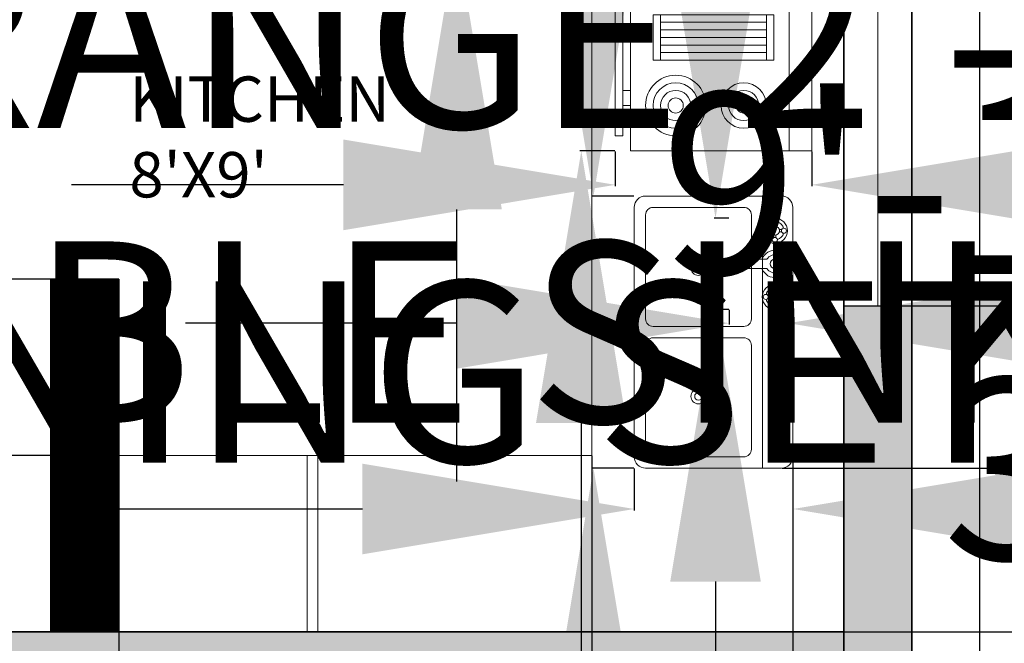
# Model space of a CAD drawing. Units: inches. Extents: x 2838 to 4029, y 1041 to 1915.
# Tile 9 of 16: x 3510 to 3640, y 1377 to 1460. Entities that reach past the tile are written whole.
import ezdxf

# ---------------------------------------------------------------- set-up
doc = ezdxf.new("R2010")
doc.units = ezdxf.units.IN
doc.header["$MEASUREMENT"] = 0
for name, color, linetype, lineweight in [('A-ANNO-DIMS', 2, 'Continuous', 18), ('A-AREA-IDEN', 7, 'Continuous', 18), ('A-EQPM', 8, 'Continuous', 18), ('A-FLOR', 7, 'Continuous', 25), ('A-FLOR-CASE', 8, 'Continuous', 18), ('A-FLOR-FIXT', 9, 'Continuous', 18), ('A-GLAZ', 4, 'Continuous', 18), ('A-WALL', 7, 'Continuous', 35), ('A-WALL-PATT', 252, 'Continuous', 13)]:
    doc.layers.add(name, color=color, linetype=linetype, lineweight=lineweight)
doc.styles.get("Standard").update_dxf_attribs({"font": 'arial.ttf'})
doc.dimstyles.get("Standard").update_dxf_attribs({"dimtxt": 24, "dimasz": 36, "dimexe": 0.18, "dimexo": 0.0625, "dimgap": 0.09, "dimtad": 0, "dimtih": 1, "dimtoh": 1, "dimdec": 0, "dimzin": 0, "dimdsep": 46, "dimlunit": 3, "dimtxsty": 'Standard', "dimcen": 0.09, "dimadec": 0, "dimazin": 0, "dimtfac": 1, "dimtdec": 0, "dimtofl": 0, "dimtmove": 0, "dimatfit": 3, "dimfxl": 1, "dimtolj": 1, "dimtzin": 0, "dimarcsym": 0})

# ---------------------------------------------------------------- blocks, each defined once
blk = doc.blocks.new('Faucet - Bathroom top')
for p, q in [((-4.107, 0.125), (-4.375, 0.125)), ((-3.75, 0.4788), (-3.75, 0.75)), ((-3.5, 0.482), (-3.5, 0.75)), ((-3.1461, 0.125), (-2.875, 0.125)), ((3.143, 0.125), (2.875, 0.125)), ((3.5, 0.4788), (3.5, 0.75)), ((3.75, 0.482), (3.75, 0.75)), ((4.1039, 0.125), (4.375, 0.125)), ((-4.1039, -0.125), (-4.375, -0.125)), ((-3.75, -0.4821), (-3.75, -0.75)), ((-3.5, -0.4789), (-3.5, -0.75)), ((-3.143, -0.125), (-2.875, -0.125)), ((-0.5, -0.8639), (-0.5, -4.5)), ((0.5, -4.5), (0.5, -0.8631)), ((3.1461, -0.125), (2.875, -0.125)), ((3.5, -0.4821), (3.5, -0.75)), ((3.75, -0.4789), (3.75, -0.75)), ((4.107, -0.125), (4.375, -0.125))]:
    blk.add_line(p, q)
for centre, radius in [((-3.625, 0), 1.375), ((-3.625, 1), 0.2795), ((3.625, 0), 1.375), ((3.625, 1), 0.2795), ((-4.625, 0), 0.2795), ((-3.625, 0), 0.5), ((-2.625, 0), 0.2795), ((0, 0), 0.5), ((2.625, 0), 0.2795), ((3.625, 0), 0.5), ((4.625, 0), 0.2795), ((-3.625, -1), 0.2795), ((3.625, -1), 0.2795)]:
    blk.add_circle(centre, radius)
for centre, radius, start, end in [((0, 0), 1.5, 289.6514, 250.3603), ((-3.625, 0), 1, 105.2407, 164.2093), ((-3.625, 0), 1, 16.44125, 74.07887), ((0, 0), 1, 300.3431, 239.7554), ((3.625, 0), 1, 106.12, 164.0884), ((3.625, 0), 1, 16.23422, 73.90469), ((-3.625, 0), 1, 196.2342, 253.9047), ((-3.625, 0), 1, 286.12, 344.0884), ((3.625, 0), 1, 196.4413, 254.0789), ((3.625, 0), 1, 285.2407, 344.2093), ((0, -4.5), 0.5, 180, 0)]:
    blk.add_arc(centre, radius, start, end)
blk = doc.blocks.new('Range-Oven - 30 in top')
for p, q in [((0, -3), (30, -3)), ((12, -6), (18, -6)), ((13, -20), (13, -6)), ((14, -6), (14, -20)), ((15, -20), (15, -6)), ((16, -6), (16, -20)), ((17, -20), (17, -6)), ((18, -20), (12, -20)), ((6, -24), (6, -25)), ((8, -25), (8, -24)), ((22, -25), (22, -24)), ((24, -24), (24, -25))]:
    blk.add_line(p, q)
for points in [[(0, -24), (0, 0), (30, 0), (30, -24)], [(12, -21), (12, -5), (18, -5), (18, -21)], [(2, -26), (2, -25), (28, -25), (28, -26)]]:
    blk.add_lwpolyline(points, close=True)
for centre, radius in [((6, -9), 4), ((6, -9), 3), ((24, -9), 3), ((6, -9), 2), ((24, -9), 2), ((6, -9), 1), ((24, -9), 1), ((24, -18), 4), ((6, -18), 3), ((24, -18), 3), ((6, -18), 2), ((24, -18), 2), ((6, -18), 1), ((24, -18), 1)]:
    blk.add_circle(centre, radius)
blk = doc.blocks.new('Sink-double - 36 in top')
for p, q in [((-18, -4), (18, -4)), ((-0.75, -18.5), (-0.75, -6.5)), ((0.75, -6.5), (0.75, -18.5))]:
    blk.add_line(p, q)
for points in [[(-16.5, 0), (16.5, 0)], [(-18, -19.5), (-18, -1.5)], [(18, -1.5), (18, -19.5)], [(-16.5, -18.5), (-16.5, -6.5)], [(-15.5, -5.5), (-1.75, -5.5)], [(1.75, -5.5), (15.5, -5.5)], [(16.5, -6.5), (16.5, -18.5)], [(-1.75, -19.5), (-15.5, -19.5)], [(15.5, -19.5), (1.75, -19.5)], [(16.5, -21), (-16.5, -21)]]:
    blk.add_lwpolyline(points)
for centre, radius in [((-8.5, -12.5), 1), ((8.5, -12.5), 1), ((-8.5, -12.5), 0.5), ((8.5, -12.5), 0.5)]:
    blk.add_circle(centre, radius)
for centre, radius, start, end in [((-16.5, -1.5), 1.5, 90, 180), ((16.5, -1.5), 1.5, 0, 90), ((-15.5, -6.5), 1, 90, 180), ((-1.75, -6.5), 1, 0, 90), ((1.75, -6.5), 1, 90, 180), ((15.5, -6.5), 1, 0, 90), ((-16.5, -19.5), 1.5, 180, 270), ((-15.5, -18.5), 1, 180, 270), ((-1.75, -18.5), 1, 270, 0), ((1.75, -18.5), 1, 180, 270), ((15.5, -18.5), 1, 270, 0), ((16.5, -19.5), 1.5, 270, 0)]:
    blk.add_arc(centre, radius, start, end)
blk = doc.blocks.new('*D17')
at = {"layer": 'A-ANNO-DIMS', "color": 0, "lineweight": -2, "transparency": 16777216}
for p, q in [((3627.79, 1671.3), (3713.18, 1671.3)), ((3713, 1635.3), (3713, 1443.64)), ((3713, 1227.3), (3713, 1418.95)), ((3627.79, 1191.3), (3713.18, 1191.3))]:
    blk.add_line(p, q, dxfattribs=at)
at = {"layer": 'A-ANNO-DIMS', "color": 0, "transparency": 16777216}
for points in [[(3707, 1635.3), (3719, 1635.3), (3713, 1671.3)], [(3707, 1227.3), (3719, 1227.3), (3713, 1191.3)]]:
    blk.add_solid(points, dxfattribs=at)
at = {"layer": 'Defpoints', "color": 0, "transparency": 16777216}
for p in [(3627.73, 1671.3), (3627.73, 1191.3), (3713, 1191.3)]:
    blk.add_point(p, dxfattribs=at)
at = {"layer": 'A-ANNO-DIMS', "color": 0, "transparency": 16777216, "insert": (3713, 1431.3), "char_height": 24, "attachment_point": 5}
blk.add_mtext("\\A1;40'", dxfattribs=at)
blk = doc.blocks.new('WIN-48')
blk.add_line((4.5, 48), (4.5, 0))
blk.add_lwpolyline([(0, 48), (9, 48), (9, 0), (0, 0)], close=True)
blk = doc.blocks.new('*D33')
at = {"layer": 'A-ANNO-DIMS', "color": 0, "lineweight": -2, "transparency": 16777216}
for p, q in [((3601.73, 1469.45), (3601.73, 1505.45)), ((3603.48, 1433.45), (3601.55, 1433.45)), ((3603.48, 1421.37), (3601.55, 1421.37)), ((3601.73, 1385.37), (3601.73, 1349.37)), ((3601.73, 1349.37), (3565.73, 1349.37))]:
    blk.add_line(p, q, dxfattribs=at)
at = {"layer": 'A-ANNO-DIMS', "color": 0, "transparency": 16777216}
for points in [[(3595.73, 1469.45), (3607.73, 1469.45), (3601.73, 1433.45)], [(3595.73, 1385.37), (3607.73, 1385.37), (3601.73, 1421.37)]]:
    blk.add_solid(points, dxfattribs=at)
at = {"layer": 'Defpoints', "color": 0, "transparency": 16777216}
for p in [(3603.54, 1433.45), (3601.73, 1421.37), (3603.54, 1421.37)]:
    blk.add_point(p, dxfattribs=at)
at = {"layer": 'A-ANNO-DIMS', "color": 0, "transparency": 16777216, "insert": (3496.18, 1349.37), "char_height": 24, "attachment_point": 5}
blk.add_mtext('\\A1;TAP 1\'-0"', dxfattribs=at)
blk = doc.blocks.new('*D34')
at = {"layer": 'A-ANNO-DIMS', "color": 0, "lineweight": -2, "transparency": 16777216}
for p, q in [((3603.54, 1421.31), (3603.54, 1419.38)), ((3611.39, 1421.31), (3611.39, 1419.38)), ((3567.54, 1419.56), (3531.54, 1419.56)), ((3647.39, 1419.56), (3683.39, 1419.56))]:
    blk.add_line(p, q, dxfattribs=at)
at = {"layer": 'A-ANNO-DIMS', "color": 0, "transparency": 16777216}
for points in [[(3567.54, 1425.56), (3567.54, 1413.56), (3603.54, 1419.56)], [(3647.39, 1425.56), (3647.39, 1413.56), (3611.39, 1419.56)]]:
    blk.add_solid(points, dxfattribs=at)
at = {"layer": 'Defpoints', "color": 0, "transparency": 16777216}
for p in [(3603.54, 1421.37), (3611.39, 1421.37), (3611.39, 1419.56)]:
    blk.add_point(p, dxfattribs=at)
at = {"layer": 'A-ANNO-DIMS', "color": 0, "transparency": 16777216, "insert": (3715.38, 1419.56), "char_height": 24, "attachment_point": 5}
blk.add_mtext('\\A1;0\'-8"', dxfattribs=at)
blk = doc.blocks.new('*D41')
at = {"layer": 'A-ANNO-DIMS', "color": 0, "lineweight": -2, "transparency": 16777216}
for p, q in [((3284.24, 1506.2), (3284.24, 1496.56)), ((3347.73, 1506.2), (3347.73, 1496.56)), ((3248.24, 1496.74), (3212.24, 1496.74)), ((3383.73, 1496.74), (3419.73, 1496.74))]:
    blk.add_line(p, q, dxfattribs=at)
at = {"layer": 'A-ANNO-DIMS', "color": 0, "transparency": 16777216}
for points in [[(3248.24, 1502.74), (3248.24, 1490.74), (3284.24, 1496.74)], [(3383.73, 1502.74), (3383.73, 1490.74), (3347.73, 1496.74)]]:
    blk.add_solid(points, dxfattribs=at)
at = {"layer": 'Defpoints', "color": 0, "transparency": 16777216}
for p in [(3284.24, 1506.26), (3347.73, 1506.26), (3347.73, 1496.74)]:
    blk.add_point(p, dxfattribs=at)
at = {"layer": 'A-ANNO-DIMS', "color": 0, "transparency": 16777216, "insert": (3624.81, 1496.74), "char_height": 24, "attachment_point": 5}
blk.add_mtext('\\A1;WARDROBE 5\'-3 1/2" TYP.', dxfattribs=at)
blk = doc.blocks.new('*D49')
at = {"layer": 'A-ANNO-DIMS', "color": 0, "lineweight": -2, "transparency": 16777216}
for p, q in [((3336.37, 1426.68), (3336.37, 1412.92)), ((3427.37, 1426.68), (3427.37, 1412.92)), ((3372.37, 1413.1), (3391.37, 1413.1)), ((3427.37, 1413.1), (3463.37, 1413.1))]:
    blk.add_line(p, q, dxfattribs=at)
at = {"layer": 'A-ANNO-DIMS', "color": 0, "transparency": 16777216}
for points in [[(3372.37, 1419.1), (3372.37, 1407.1), (3336.37, 1413.1)], [(3391.37, 1419.1), (3391.37, 1407.1), (3427.37, 1413.1)]]:
    blk.add_solid(points, dxfattribs=at)
at = {"layer": 'Defpoints', "color": 0, "transparency": 16777216}
for p in [(3336.37, 1426.75), (3427.37, 1426.75), (3427.37, 1413.1)]:
    blk.add_point(p, dxfattribs=at)
at = {"layer": 'A-ANNO-DIMS', "color": 0, "transparency": 16777216, "insert": (3595.36, 1413.1), "char_height": 24, "attachment_point": 5}
blk.add_mtext('\\A1;DINING SET 7\'-7"', dxfattribs=at)
blk = doc.blocks.new('*D53')
at = {"layer": 'A-ANNO-DIMS', "color": 0, "lineweight": -2, "transparency": 16777216}
for p, q in [((3583.96, 1508.36), (3583.96, 1544.36)), ((3588.4, 1472.36), (3583.78, 1472.36)), ((3588.4, 1442.36), (3583.78, 1442.36)), ((3583.96, 1406.36), (3583.96, 1370.36))]:
    blk.add_line(p, q, dxfattribs=at)
at = {"layer": 'A-ANNO-DIMS', "color": 0, "transparency": 16777216}
for points in [[(3577.96, 1508.36), (3589.96, 1508.36), (3583.96, 1472.36)], [(3577.96, 1406.36), (3589.96, 1406.36), (3583.96, 1442.36)]]:
    blk.add_solid(points, dxfattribs=at)
at = {"layer": 'Defpoints', "color": 0, "transparency": 16777216}
for p in [(3588.46, 1472.36), (3583.96, 1442.36), (3588.46, 1442.36)]:
    blk.add_point(p, dxfattribs=at)
at = {"layer": 'A-ANNO-DIMS', "color": 0, "transparency": 16777216, "insert": (3583.96, 1457.36), "char_height": 24, "attachment_point": 5}
blk.add_mtext('\\A1;RANGE 2\'-6"', dxfattribs=at)
blk = doc.blocks.new('*D54')
at = {"layer": 'A-ANNO-DIMS', "color": 0, "lineweight": -2, "transparency": 16777216}
for p, q in [((3588.46, 1442.29), (3588.46, 1437.68)), ((3614.46, 1442.29), (3614.46, 1437.68)), ((3552.46, 1437.86), (3516.46, 1437.86)), ((3650.46, 1437.86), (3686.46, 1437.86))]:
    blk.add_line(p, q, dxfattribs=at)
at = {"layer": 'A-ANNO-DIMS', "color": 0, "transparency": 16777216}
for points in [[(3552.46, 1443.86), (3552.46, 1431.86), (3588.46, 1437.86)], [(3650.46, 1443.86), (3650.46, 1431.86), (3614.46, 1437.86)]]:
    blk.add_solid(points, dxfattribs=at)
at = {"layer": 'Defpoints', "color": 0, "transparency": 16777216}
for p in [(3588.46, 1442.36), (3614.46, 1442.36), (3614.46, 1437.86)]:
    blk.add_point(p, dxfattribs=at)
at = {"layer": 'A-ANNO-DIMS', "color": 0, "transparency": 16777216, "insert": (3718.65, 1437.86), "char_height": 24, "attachment_point": 5}
blk.add_mtext('\\A1;2\'-2"', dxfattribs=at)
blk = doc.blocks.new('*D55')
at = {"layer": 'A-ANNO-DIMS', "color": 0, "lineweight": -2, "transparency": 16777216}
for p, q in [((3491.76, 1499.78), (3455.76, 1499.78)), ((3527.76, 1494.67), (3527.76, 1499.96)), ((3562.26, 1494.67), (3562.26, 1499.96)), ((3598.26, 1499.78), (3634.26, 1499.78))]:
    blk.add_line(p, q, dxfattribs=at)
at = {"layer": 'A-ANNO-DIMS', "color": 0, "transparency": 16777216}
for points in [[(3491.76, 1505.78), (3491.76, 1493.78), (3527.76, 1499.78)], [(3598.26, 1505.78), (3598.26, 1493.78), (3562.26, 1499.78)]]:
    blk.add_solid(points, dxfattribs=at)
at = {"layer": 'Defpoints', "color": 0, "transparency": 16777216}
for p in [(3527.76, 1499.78), (3527.76, 1494.6), (3562.26, 1494.6)]:
    blk.add_point(p, dxfattribs=at)
at = {"layer": 'A-ANNO-DIMS', "color": 0, "transparency": 16777216, "insert": (3260.33, 1499.78), "char_height": 24, "attachment_point": 5}
blk.add_mtext('\\A1;BASE CABINET 2\'-10 1/2"', dxfattribs=at)
blk = doc.blocks.new('*D56')
at = {"layer": 'A-ANNO-DIMS', "color": 0, "lineweight": -2, "transparency": 16777216}
for p, q in [((3567.44, 1530.6), (3567.44, 1566.6)), ((3567.44, 1566.6), (3603.44, 1566.6)), ((3562.33, 1494.6), (3567.62, 1494.6)), ((3562.33, 1470.6), (3567.62, 1470.6)), ((3567.44, 1434.6), (3567.44, 1398.6))]:
    blk.add_line(p, q, dxfattribs=at)
at = {"layer": 'A-ANNO-DIMS', "color": 0, "transparency": 16777216}
for points in [[(3561.44, 1530.6), (3573.44, 1530.6), (3567.44, 1494.6)], [(3561.44, 1434.6), (3573.44, 1434.6), (3567.44, 1470.6)]]:
    blk.add_solid(points, dxfattribs=at)
at = {"layer": 'Defpoints', "color": 0, "transparency": 16777216}
for p in [(3562.26, 1494.6), (3567.44, 1494.6), (3562.26, 1470.6)]:
    blk.add_point(p, dxfattribs=at)
at = {"layer": 'A-ANNO-DIMS', "color": 0, "transparency": 16777216, "insert": (3635.63, 1566.6), "char_height": 24, "attachment_point": 5}
blk.add_mtext('\\A1;2\'-0"', dxfattribs=at)
blk = doc.blocks.new('*D57')
at = {"layer": 'A-ANNO-DIMS', "color": 0, "lineweight": -2, "transparency": 16777216}
for p, q in [((3585.57, 1472.38), (3585.57, 1508.38)), ((3590.9, 1436.38), (3585.39, 1436.38)), ((3590.9, 1400.38), (3585.39, 1400.38)), ((3585.57, 1364.38), (3585.57, 1328.38))]:
    blk.add_line(p, q, dxfattribs=at)
at = {"layer": 'A-ANNO-DIMS', "color": 0, "transparency": 16777216}
for points in [[(3579.57, 1472.38), (3591.57, 1472.38), (3585.57, 1436.38)], [(3579.57, 1364.38), (3591.57, 1364.38), (3585.57, 1400.38)]]:
    blk.add_solid(points, dxfattribs=at)
at = {"layer": 'Defpoints', "color": 0, "transparency": 16777216}
for p in [(3590.97, 1436.38), (3585.57, 1400.38), (3590.97, 1400.38)]:
    blk.add_point(p, dxfattribs=at)
at = {"layer": 'A-ANNO-DIMS', "color": 0, "transparency": 16777216, "insert": (3585.57, 1418.38), "char_height": 24, "attachment_point": 5}
blk.add_mtext('\\A1;DOUBLE SINK 3\'-0"', dxfattribs=at)
blk = doc.blocks.new('*D58')
at = {"layer": 'A-ANNO-DIMS', "color": 0, "lineweight": -2, "transparency": 16777216}
for p, q in [((3590.97, 1400.32), (3590.97, 1394.8)), ((3611.97, 1400.32), (3611.97, 1394.8)), ((3554.97, 1394.98), (3518.97, 1394.98)), ((3647.97, 1394.98), (3683.97, 1394.98))]:
    blk.add_line(p, q, dxfattribs=at)
at = {"layer": 'A-ANNO-DIMS', "color": 0, "transparency": 16777216}
for points in [[(3554.97, 1400.98), (3554.97, 1388.98), (3590.97, 1394.98)], [(3647.97, 1400.98), (3647.97, 1388.98), (3611.97, 1394.98)]]:
    blk.add_solid(points, dxfattribs=at)
at = {"layer": 'Defpoints', "color": 0, "transparency": 16777216}
for p in [(3590.97, 1400.38), (3611.97, 1400.38), (3611.97, 1394.98)]:
    blk.add_point(p, dxfattribs=at)
at = {"layer": 'A-ANNO-DIMS', "color": 0, "transparency": 16777216, "insert": (3714.83, 1394.98), "char_height": 24, "attachment_point": 5}
blk.add_mtext('\\A1;1\'-9"', dxfattribs=at)
blk = doc.blocks.new('*D73')
at = {"layer": 'A-ANNO-DIMS', "color": 0, "lineweight": -2, "transparency": 16777216}
for p, q in [((3461.038746, 1200.359846), (3461.038746, 1711.702346)), ((3618.731626, 1200.359846), (3618.731626, 1711.702346)), ((3425.038746, 1711.522346), (3389.038746, 1711.522346)), ((3654.731626, 1711.522346), (3690.731626, 1711.522346))]:
    blk.add_line(p, q, dxfattribs=at)
at = {"layer": 'A-ANNO-DIMS', "color": 0, "transparency": 16777216}
for points in [[(3425.038746, 1717.522346), (3425.038746, 1705.522346), (3461.038746, 1711.522346)], [(3654.731626, 1717.522346), (3654.731626, 1705.522346), (3618.731626, 1711.522346)]]:
    blk.add_solid(points, dxfattribs=at)
at = {"layer": 'Defpoints', "color": 0, "transparency": 16777216}
for p in [(3618.731626, 1711.522346), (3461.038746, 1200.297346), (3618.731626, 1200.297346)]:
    blk.add_point(p, dxfattribs=at)
at = {"layer": 'A-ANNO-DIMS', "color": 0, "transparency": 16777216, "insert": (3539.885186, 1711.522346), "char_height": 24, "attachment_point": 5}
blk.add_mtext('\\A1;13\'-1 1/2"', dxfattribs=at)
blk = doc.blocks.new('*D75')
at = {"layer": 'A-ANNO-DIMS', "color": 0, "lineweight": -2, "transparency": 16777216}
for p, q in [((3667.956626, 1405.727214), (3667.956626, 1441.727214)), ((3618.794126, 1369.727214), (3668.136626, 1369.727214)), ((3618.794126, 1333.727214), (3668.136626, 1333.727214)), ((3667.956626, 1297.727214), (3667.956626, 1261.727214))]:
    blk.add_line(p, q, dxfattribs=at)
at = {"layer": 'A-ANNO-DIMS', "color": 0, "transparency": 16777216}
for points in [[(3661.956626, 1405.727214), (3673.956626, 1405.727214), (3667.956626, 1369.727214)], [(3661.956626, 1297.727214), (3673.956626, 1297.727214), (3667.956626, 1333.727214)]]:
    blk.add_solid(points, dxfattribs=at)
at = {"layer": 'Defpoints', "color": 0, "transparency": 16777216}
for p in [(3618.731626, 1369.727214), (3667.956626, 1369.727214), (3618.731626, 1333.727214)]:
    blk.add_point(p, dxfattribs=at)
at = {"layer": 'A-ANNO-DIMS', "color": 0, "transparency": 16777216, "insert": (3667.956626, 1351.727214), "char_height": 24, "attachment_point": 5}
blk.add_mtext('\\A1;3\'-0"', dxfattribs=at)
blk = doc.blocks.new('*D78')
at = {"layer": 'A-ANNO-DIMS', "color": 0, "lineweight": -2, "transparency": 16777216}
for p, q in [((3667.956626, 1590.394218), (3667.956626, 1626.394218)), ((3498.794126, 1554.394218), (3668.136626, 1554.394218)), ((3498.638013, 1506.394218), (3668.136626, 1506.394218)), ((3667.956626, 1470.394218), (3667.956626, 1434.394218))]:
    blk.add_line(p, q, dxfattribs=at)
at = {"layer": 'A-ANNO-DIMS', "color": 0, "transparency": 16777216}
for points in [[(3661.956626, 1590.394218), (3673.956626, 1590.394218), (3667.956626, 1554.394218)], [(3661.956626, 1470.394218), (3673.956626, 1470.394218), (3667.956626, 1506.394218)]]:
    blk.add_solid(points, dxfattribs=at)
at = {"layer": 'Defpoints', "color": 0, "transparency": 16777216}
for p in [(3498.731626, 1554.394218), (3667.956626, 1554.394218), (3498.575513, 1506.394218)]:
    blk.add_point(p, dxfattribs=at)
at = {"layer": 'A-ANNO-DIMS', "color": 0, "transparency": 16777216, "insert": (3667.956626, 1530.394218), "char_height": 24, "attachment_point": 5}
blk.add_mtext('\\A1;4\'-0"', dxfattribs=at)
blk = doc.blocks.new('*D79')
at = {"layer": 'A-ANNO-DIMS', "color": 0, "lineweight": -2, "transparency": 16777216}
for p, q in [((3379.05, 1400.64), (3379.05, 1711.7)), ((3454.63, 1398.31), (3454.63, 1711.7)), ((3415.05, 1711.52), (3418.63, 1711.52)), ((3454.63, 1711.52), (3490.63, 1711.52))]:
    blk.add_line(p, q, dxfattribs=at)
at = {"layer": 'A-ANNO-DIMS', "color": 0, "transparency": 16777216}
for points in [[(3415.05, 1717.52), (3415.05, 1705.52), (3379.05, 1711.52)], [(3418.63, 1717.52), (3418.63, 1705.52), (3454.63, 1711.52)]]:
    blk.add_solid(points, dxfattribs=at)
at = {"layer": 'Defpoints', "color": 0, "transparency": 16777216}
for p in [(3454.63, 1711.52), (3379.05, 1400.57), (3454.63, 1398.25)]:
    blk.add_point(p, dxfattribs=at)
at = {"layer": 'A-ANNO-DIMS', "color": 0, "transparency": 16777216, "insert": (3550.65, 1711.52), "char_height": 24, "attachment_point": 5}
blk.add_mtext('\\A1;6\'-3 1/2"', dxfattribs=at)
blk = doc.blocks.new('*D82')
at = {"layer": 'A-ANNO-DIMS', "color": 0, "lineweight": -2, "transparency": 16777216}
for p, q in [((3405.73, 1573.06), (3405.73, 1081.89)), ((3441.73, 1569.23), (3441.73, 1081.89)), ((3369.73, 1082.07), (3333.73, 1082.07)), ((3477.73, 1082.07), (3513.73, 1082.07))]:
    blk.add_line(p, q, dxfattribs=at)
at = {"layer": 'A-ANNO-DIMS', "color": 0, "transparency": 16777216}
for points in [[(3369.73, 1088.07), (3369.73, 1076.07), (3405.73, 1082.07)], [(3477.73, 1088.07), (3477.73, 1076.07), (3441.73, 1082.07)]]:
    blk.add_solid(points, dxfattribs=at)
at = {"layer": 'Defpoints', "color": 0, "transparency": 16777216}
for p in [(3405.73, 1573.12), (3441.73, 1569.3), (3441.73, 1082.07)]:
    blk.add_point(p, dxfattribs=at)
at = {"layer": 'A-ANNO-DIMS', "color": 0, "transparency": 16777216, "insert": (3545.71, 1082.07), "char_height": 24, "attachment_point": 5}
blk.add_mtext('\\A1;3\'-0"', dxfattribs=at)
blk = doc.blocks.new('*D87')
at = {"layer": 'A-ANNO-DIMS', "color": 0, "lineweight": -2, "transparency": 16777216}
for p, q in [((3227.506626, 1497.394218), (3227.506626, 1533.394218)), ((3513.669126, 1461.394218), (3227.326626, 1461.394218)), ((3513.669126, 1425.394218), (3227.326626, 1425.394218)), ((3227.506626, 1389.394218), (3227.506626, 1353.394218))]:
    blk.add_line(p, q, dxfattribs=at)
at = {"layer": 'A-ANNO-DIMS', "color": 0, "transparency": 16777216}
for points in [[(3221.506626, 1497.394218), (3233.506626, 1497.394218), (3227.506626, 1461.394218)], [(3221.506626, 1389.394218), (3233.506626, 1389.394218), (3227.506626, 1425.394218)]]:
    blk.add_solid(points, dxfattribs=at)
at = {"layer": 'Defpoints', "color": 0, "transparency": 16777216}
for p in [(3227.506626, 1461.394218), (3513.731626, 1461.394218), (3513.731626, 1425.394218)]:
    blk.add_point(p, dxfattribs=at)
at = {"layer": 'A-ANNO-DIMS', "color": 0, "transparency": 16777216, "insert": (3227.506626, 1443.394218), "char_height": 24, "attachment_point": 5}
blk.add_mtext('\\A1;3\'-0"', dxfattribs=at)
blk = doc.blocks.new('*D88')
at = {"layer": 'A-ANNO-DIMS', "color": 0, "lineweight": -2, "transparency": 16777216}
for p, q in [((3522.73, 1378.66), (3522.73, 1081.89)), ((3618.73, 1378.66), (3618.73, 1081.89)), ((3558.73, 1082.07), (3582.73, 1082.07)), ((3618.73, 1082.07), (3654.73, 1082.07))]:
    blk.add_line(p, q, dxfattribs=at)
at = {"layer": 'A-ANNO-DIMS', "color": 0, "transparency": 16777216}
for points in [[(3558.73, 1088.07), (3558.73, 1076.07), (3522.73, 1082.07)], [(3582.73, 1088.07), (3582.73, 1076.07), (3618.73, 1082.07)]]:
    blk.add_solid(points, dxfattribs=at)
at = {"layer": 'Defpoints', "color": 0, "transparency": 16777216}
for p in [(3522.73, 1378.73), (3618.73, 1378.73), (3618.73, 1082.07)]:
    blk.add_point(p, dxfattribs=at)
at = {"layer": 'A-ANNO-DIMS', "color": 0, "transparency": 16777216, "insert": (3686.74, 1082.07), "char_height": 24, "attachment_point": 5}
blk.add_mtext('\\A1;8\'-0"', dxfattribs=at)
blk = doc.blocks.new('*D89')
at = {"layer": 'A-ANNO-DIMS', "color": 0, "lineweight": -2, "transparency": 16777216}
for p, q in [((3618.79, 1497.39), (3668.14, 1497.39)), ((3667.96, 1461.39), (3667.96, 1450.56)), ((3667.96, 1414.73), (3667.96, 1425.56)), ((3618.79, 1378.73), (3668.14, 1378.73))]:
    blk.add_line(p, q, dxfattribs=at)
at = {"layer": 'A-ANNO-DIMS', "color": 0, "transparency": 16777216}
for points in [[(3661.96, 1461.39), (3673.96, 1461.39), (3667.96, 1497.39)], [(3661.96, 1414.73), (3673.96, 1414.73), (3667.96, 1378.73)]]:
    blk.add_solid(points, dxfattribs=at)
at = {"layer": 'Defpoints', "color": 0, "transparency": 16777216}
for p in [(3618.73, 1497.39), (3667.96, 1497.39), (3618.73, 1378.73)]:
    blk.add_point(p, dxfattribs=at)
at = {"layer": 'A-ANNO-DIMS', "color": 0, "transparency": 16777216, "insert": (3667.96, 1438.06), "char_height": 24, "attachment_point": 5}
blk.add_mtext('\\A1;9\'-10 1/2"', dxfattribs=at)
blk = doc.blocks.new('*D90')
at = {"layer": 'A-ANNO-DIMS', "color": 0, "lineweight": -2, "transparency": 16777216}
for p, q in [((3667.96, 1457.85), (3667.96, 1493.85)), ((3618.79, 1421.85), (3668.14, 1421.85)), ((3618.79, 1378.73), (3668.14, 1378.73)), ((3667.96, 1342.73), (3667.96, 1306.73))]:
    blk.add_line(p, q, dxfattribs=at)
at = {"layer": 'A-ANNO-DIMS', "color": 0, "transparency": 16777216}
for points in [[(3661.96, 1457.85), (3673.96, 1457.85), (3667.96, 1421.85)], [(3661.96, 1342.73), (3673.96, 1342.73), (3667.96, 1378.73)]]:
    blk.add_solid(points, dxfattribs=at)
at = {"layer": 'Defpoints', "color": 0, "transparency": 16777216}
for p in [(3618.73, 1421.85), (3667.96, 1421.85), (3618.73, 1378.73)]:
    blk.add_point(p, dxfattribs=at)
at = {"layer": 'A-ANNO-DIMS', "color": 0, "transparency": 16777216, "insert": (3667.96, 1400.29), "char_height": 24, "attachment_point": 5}
blk.add_mtext('\\A1;3\'-7"', dxfattribs=at)
blk = doc.blocks.new('*D91')
at = {"layer": 'A-ANNO-DIMS', "color": 0, "lineweight": -2, "transparency": 16777216}
for p, q in [((3227.506626, 1533.394218), (3227.506626, 1569.394218)), ((3522.669126, 1497.394218), (3227.326626, 1497.394218)), ((3522.669126, 1461.394218), (3227.326626, 1461.394218)), ((3227.506626, 1425.394218), (3227.506626, 1389.394218))]:
    blk.add_line(p, q, dxfattribs=at)
at = {"layer": 'A-ANNO-DIMS', "color": 0, "transparency": 16777216}
for points in [[(3221.506626, 1533.394218), (3233.506626, 1533.394218), (3227.506626, 1497.394218)], [(3221.506626, 1425.394218), (3233.506626, 1425.394218), (3227.506626, 1461.394218)]]:
    blk.add_solid(points, dxfattribs=at)
at = {"layer": 'Defpoints', "color": 0, "transparency": 16777216}
for p in [(3522.731626, 1497.394218), (3227.506626, 1461.394218), (3522.731626, 1461.394218)]:
    blk.add_point(p, dxfattribs=at)
at = {"layer": 'A-ANNO-DIMS', "color": 0, "transparency": 16777216, "insert": (3227.506626, 1479.394218), "char_height": 24, "attachment_point": 5}
blk.add_mtext('\\A1;3\'-0"', dxfattribs=at)
blk = doc.blocks.new('*D92')
at = {"layer": 'A-ANNO-DIMS', "color": 0, "lineweight": -2, "transparency": 16777216}
for p, q in [((3585.37, 1402), (3585.37, 1081.89)), ((3618.73, 1378.66), (3618.73, 1081.89)), ((3549.37, 1082.07), (3513.37, 1082.07)), ((3654.73, 1082.07), (3690.73, 1082.07))]:
    blk.add_line(p, q, dxfattribs=at)
at = {"layer": 'A-ANNO-DIMS', "color": 0, "transparency": 16777216}
for points in [[(3549.37, 1088.07), (3549.37, 1076.07), (3585.37, 1082.07)], [(3654.73, 1088.07), (3654.73, 1076.07), (3618.73, 1082.07)]]:
    blk.add_solid(points, dxfattribs=at)
at = {"layer": 'Defpoints', "color": 0, "transparency": 16777216}
for p in [(3585.37, 1402.06), (3618.73, 1378.73), (3618.73, 1082.07)]:
    blk.add_point(p, dxfattribs=at)
at = {"layer": 'A-ANNO-DIMS', "color": 0, "transparency": 16777216, "insert": (3750.89, 1082.07), "char_height": 24, "attachment_point": 5}
blk.add_mtext('\\A1;2\'-9 1/2"', dxfattribs=at)
blk = doc.blocks.new('*D93')
at = {"layer": 'A-ANNO-DIMS', "color": 0, "lineweight": -2, "transparency": 16777216}
for p, q in [((3227.51, 1438.06), (3227.51, 1474.06)), ((3227.51, 1474.06), (3263.51, 1474.06)), ((3522.67, 1402.06), (3227.33, 1402.06)), ((3522.67, 1378.73), (3227.33, 1378.73)), ((3227.51, 1342.73), (3227.51, 1306.73))]:
    blk.add_line(p, q, dxfattribs=at)
at = {"layer": 'A-ANNO-DIMS', "color": 0, "transparency": 16777216}
for points in [[(3221.51, 1438.06), (3233.51, 1438.06), (3227.51, 1402.06)], [(3221.51, 1342.73), (3233.51, 1342.73), (3227.51, 1378.73)]]:
    blk.add_solid(points, dxfattribs=at)
at = {"layer": 'Defpoints', "color": 0, "transparency": 16777216}
for p in [(3227.51, 1402.06), (3522.73, 1402.06), (3522.73, 1378.73)]:
    blk.add_point(p, dxfattribs=at)
at = {"layer": 'A-ANNO-DIMS', "color": 0, "transparency": 16777216, "insert": (3331.65, 1474.06), "char_height": 24, "attachment_point": 5}
blk.add_mtext('\\A1;1\'-11 1/2"', dxfattribs=at)
blk = doc.blocks.new('*D94')
at = {"layer": 'A-ANNO-DIMS', "color": 0, "lineweight": -2, "transparency": 16777216}
for p, q in [((3667.96, 1533.39), (3667.96, 1569.39)), ((3585.44, 1497.39), (3668.14, 1497.39)), ((3585.44, 1469.25), (3668.14, 1469.25)), ((3667.96, 1433.25), (3667.96, 1397.25))]:
    blk.add_line(p, q, dxfattribs=at)
at = {"layer": 'A-ANNO-DIMS', "color": 0, "transparency": 16777216}
for points in [[(3661.96, 1533.39), (3673.96, 1533.39), (3667.96, 1497.39)], [(3661.96, 1433.25), (3673.96, 1433.25), (3667.96, 1469.25)]]:
    blk.add_solid(points, dxfattribs=at)
at = {"layer": 'Defpoints', "color": 0, "transparency": 16777216}
for p in [(3585.37, 1497.39), (3585.37, 1469.25), (3667.96, 1469.25)]:
    blk.add_point(p, dxfattribs=at)
at = {"layer": 'A-ANNO-DIMS', "color": 0, "transparency": 16777216, "insert": (3667.96, 1483.32), "char_height": 24, "attachment_point": 5}
blk.add_mtext('\\A1;2\'-4"', dxfattribs=at)
blk = doc.blocks.new('*D101')
at = {"layer": 'A-ANNO-DIMS', "color": 0, "lineweight": -2, "transparency": 16777216}
for p, q in [((3461.04, 1200.36), (3461.04, 1711.7)), ((3486.18, 1200.36), (3486.18, 1711.7)), ((3425.04, 1711.52), (3389.04, 1711.52)), ((3522.18, 1711.52), (3558.18, 1711.52))]:
    blk.add_line(p, q, dxfattribs=at)
at = {"layer": 'A-ANNO-DIMS', "color": 0, "transparency": 16777216}
for points in [[(3425.04, 1717.52), (3425.04, 1705.52), (3461.04, 1711.52)], [(3522.18, 1717.52), (3522.18, 1705.52), (3486.18, 1711.52)]]:
    blk.add_solid(points, dxfattribs=at)
at = {"layer": 'Defpoints', "color": 0, "transparency": 16777216}
for p in [(3486.18, 1711.52), (3461.04, 1200.3), (3486.18, 1200.3)]:
    blk.add_point(p, dxfattribs=at)
at = {"layer": 'A-ANNO-DIMS', "color": 0, "transparency": 16777216, "insert": (3590.37, 1711.52), "char_height": 24, "attachment_point": 5}
blk.add_mtext('\\A1;2\'-1"', dxfattribs=at)
blk = doc.blocks.new('*D104')
at = {"layer": 'A-ANNO-DIMS', "color": 0, "lineweight": -2, "transparency": 16777216}
for p, q in [((3667.956626, 1533.394218), (3667.956626, 1569.394218)), ((3618.794126, 1497.394218), (3668.136626, 1497.394218)), ((3614.522024, 1472.357294), (3668.136626, 1472.357294)), ((3667.956626, 1436.357294), (3667.956626, 1400.357294))]:
    blk.add_line(p, q, dxfattribs=at)
at = {"layer": 'A-ANNO-DIMS', "color": 0, "transparency": 16777216}
for points in [[(3661.956626, 1533.394218), (3673.956626, 1533.394218), (3667.956626, 1497.394218)], [(3661.956626, 1436.357294), (3673.956626, 1436.357294), (3667.956626, 1472.357294)]]:
    blk.add_solid(points, dxfattribs=at)
at = {"layer": 'Defpoints', "color": 0, "transparency": 16777216}
for p in [(3618.731626, 1497.394218), (3614.459524, 1472.357294), (3667.956626, 1472.357294)]:
    blk.add_point(p, dxfattribs=at)
at = {"layer": 'A-ANNO-DIMS', "color": 0, "transparency": 16777216, "insert": (3667.956626, 1484.875756), "char_height": 24, "attachment_point": 5}
blk.add_mtext('\\A1;2\'-1"', dxfattribs=at)
blk = doc.blocks.new('*D106')
at = {"layer": 'A-ANNO-DIMS', "color": 0, "lineweight": -2, "transparency": 16777216}
for p, q in [((3611.97, 1401.82), (3611.97, 1081.89)), ((3618.73, 1378.66), (3618.73, 1081.89)), ((3575.97, 1082.07), (3539.97, 1082.07)), ((3654.73, 1082.07), (3690.73, 1082.07))]:
    blk.add_line(p, q, dxfattribs=at)
at = {"layer": 'A-ANNO-DIMS', "color": 0, "transparency": 16777216}
for points in [[(3575.97, 1088.07), (3575.97, 1076.07), (3611.97, 1082.07)], [(3654.73, 1088.07), (3654.73, 1076.07), (3618.73, 1082.07)]]:
    blk.add_solid(points, dxfattribs=at)
at = {"layer": 'Defpoints', "color": 0, "transparency": 16777216}
for p in [(3611.97, 1401.88), (3618.73, 1378.73), (3618.73, 1082.07)]:
    blk.add_point(p, dxfattribs=at)
at = {"layer": 'A-ANNO-DIMS', "color": 0, "transparency": 16777216, "insert": (3722.72, 1082.07), "char_height": 24, "attachment_point": 5}
blk.add_mtext('\\A1;0\'-7"', dxfattribs=at)
blk = doc.blocks.new('*D107')
at = {"layer": 'A-ANNO-DIMS', "color": 0, "lineweight": -2, "transparency": 16777216}
for p, q in [((3667.96, 1436.38), (3667.96, 1472.38)), ((3610.53, 1400.38), (3668.14, 1400.38)), ((3618.79, 1378.73), (3668.14, 1378.73)), ((3667.96, 1342.73), (3667.96, 1306.73)), ((3667.96, 1306.73), (3631.96, 1306.73))]:
    blk.add_line(p, q, dxfattribs=at)
at = {"layer": 'A-ANNO-DIMS', "color": 0, "transparency": 16777216}
for points in [[(3661.96, 1436.38), (3673.96, 1436.38), (3667.96, 1400.38)], [(3661.96, 1342.73), (3673.96, 1342.73), (3667.96, 1378.73)]]:
    blk.add_solid(points, dxfattribs=at)
at = {"layer": 'Defpoints', "color": 0, "transparency": 16777216}
for p in [(3610.47, 1400.38), (3618.73, 1378.73), (3667.96, 1378.73)]:
    blk.add_point(p, dxfattribs=at)
at = {"layer": 'A-ANNO-DIMS', "color": 0, "transparency": 16777216, "insert": (3573.14, 1306.73), "char_height": 24, "attachment_point": 5}
blk.add_mtext('\\A1;1\'-9 1/2"', dxfattribs=at)

msp = doc.modelspace()

# ---------------------------------------------------------------- hatches: boundary and pattern name
at = {"layer": 'A-WALL-PATT'}
h = msp.add_hatch(color=256, dxfattribs=at)
h.dxf.hatch_style = 1
h.paths.add_polyline_path([(3427.52, 1671.3), (3360.91, 1671.3), (3360.91, 1662.3), (3396.73, 1662.3), (3396.73, 1554.39), (3397.12, 1554.39, -0.007312), (3398.53, 1554.41), (3405.73, 1554.41), (3405.73, 1662.3), (3427.52, 1662.3)])
h.paths.add_polyline_path([(3546.42, 1671.3), (3451.52, 1671.3), (3451.52, 1662.3), (3489.73, 1662.3), (3489.73, 1592.86, -0.016107), (3489.73, 1591.9), (3489.73, 1578.3), (3441.73, 1578.3), (3441.73, 1569.3), (3489.73, 1569.3), (3489.73, 1554.41), (3498.73, 1554.41), (3498.73, 1662.3), (3546.42, 1662.3)])
h.paths.add_polyline_path([(3627.73, 1671.3), (3594.42, 1671.3), (3594.42, 1662.3), (3618.73, 1662.3), (3618.73, 1634.03), (3627.73, 1634.03)])
h.paths.add_polyline_path([(3627.73, 1586.03), (3618.73, 1586.03), (3618.73, 1506.39), (3545.12, 1506.39), (3489.73, 1506.39), (3489.73, 1497.39), (3513.73, 1497.39), (3618.73, 1497.39), (3618.73, 1469.85), (3627.73, 1469.85)])
h.paths.add_polyline_path([(3627.73, 1421.85), (3618.73, 1421.85), (3618.73, 1378.73), (3522.73, 1378.73), (3513.73, 1378.73), (3461.04, 1378.73), (3461.04, 1369.73), (3513.73, 1369.73), (3618.73, 1369.73), (3618.73, 1320.94), (3627.73, 1320.94)])
h.paths.add_polyline_path([(3627.73, 1272.94), (3618.73, 1272.94), (3618.73, 1200.3), (3599.07, 1200.3), (3599.07, 1191.3), (3627.73, 1191.3)])
h.paths.add_polyline_path([(3551.07, 1200.3), (3510.18, 1200.3), (3510.18, 1191.3), (3551.07, 1191.3)])
h.paths.add_polyline_path([(3486.18, 1200.3), (3461.04, 1200.3), (3461.04, 1398.25), (3454.63, 1398.25), (3454.63, 1200.3), (3432.45, 1200.3), (3432.45, 1191.3), (3486.18, 1191.3)])
h.paths.add_polyline_path([(3300.73, 1200.3), (3276.73, 1200.3), (3276.73, 1391.57), (3331.05, 1391.57), (3331.05, 1400.57), (3276.73, 1400.57), (3276.73, 1432.17), (3267.73, 1432.17), (3267.73, 1191.3), (3300.73, 1191.3)])
h = msp.add_hatch(dxfattribs=at)
h.set_pattern_fill('ANSI31', color=256)
h.paths.add_polyline_path([(3522.73, 1497.39), (3513.73, 1497.39), (3513.73, 1461.39), (3522.73, 1461.39)])
h.paths.add_polyline_path([(3522.73, 1425.39), (3513.73, 1425.39), (3513.73, 1378.73), (3522.73, 1378.73), (3522.73, 1402.06)])

# ---------------------------------------------------------------- linework, layer by layer
at = {"layer": 'A-FLOR'}
msp.add_lwpolyline([(3527.95, 1182.3), (3636.73, 1182.3), (3636.73, 1680.3), (3258.73, 1680.3), (3258.73, 1182.3), (3267.73, 1182.3)], dxfattribs=at)
at = {"layer": 'A-FLOR-CASE'}
msp.add_line((3549.1, 1402.06), (3549.1, 1378.73), dxfattribs=at)
for points in [[(3585.37, 1378.73), (3618.73, 1378.73), (3618.73, 1497.39), (3585.37, 1497.39), (3585.37, 1402.06)], [(3618.73, 1402.06), (3618.73, 1378.73), (3522.73, 1378.73), (3522.73, 1402.06), (3585.37, 1402.06)]]:
    msp.add_lwpolyline(points, dxfattribs=at)
msp.add_lwpolyline([(3522.73, 1402.06), (3547.68, 1402.06), (3547.68, 1378.73), (3522.73, 1378.73)], close=True, dxfattribs=at)
at = {"layer": 'A-WALL'}
for p, q in [((3627.73, 1191.3), (3627.73, 1671.3)), ((3627.73, 1421.85), (3627.73, 1586.03)), ((3618.73, 1378.73), (3618.73, 1497.39)), ((3618.73, 1469.85), (3618.73, 1421.85)), ((3618.73, 1421.85), (3618.73, 1469.25)), ((3618.73, 1469.25), (3618.73, 1421.85)), ((3513.73, 1378.73), (3513.73, 1425.39)), ((3522.73, 1425.39), (3513.73, 1425.39)), ((3522.73, 1378.73), (3522.73, 1425.39)), ((3618.73, 1421.85), (3618.73, 1378.73)), ((3627.73, 1320.94), (3627.73, 1421.85)), ((3513.73, 1381.73), (3513.73, 1378.73)), ((3522.73, 1381.73), (3522.73, 1378.73)), ((3522.73, 1378.73), (3522.73, 1381.73)), ((3513.73, 1378.73), (3461.04, 1378.73)), ((3513.73, 1378.73), (3461.04, 1378.73)), ((3618.73, 1378.73), (3513.73, 1378.73)), ((3522.73, 1378.73), (3513.73, 1378.73)), ((3618.73, 1378.73), (3522.73, 1378.73))]:
    msp.add_line(p, q, dxfattribs=at)
msp.add_lwpolyline([(3372.73, 1191.3), (3627.73, 1191.3), (3627.73, 1671.3), (3267.73, 1671.3), (3267.73, 1191.3), (3300.73, 1191.3)], dxfattribs=at)

# ---------------------------------------------------------------- block references
at = {"layer": 'A-EQPM', "rotation": 270}
msp.add_blockref('Range-Oven - 30 in top', (3614.46, 1472.36), dxfattribs=at)
at = {"layer": 'A-FLOR-FIXT', "rotation": 270}
msp.add_blockref('Sink-double - 36 in top', (3611.97, 1418.38), dxfattribs=at)
at = {"layer": 'A-FLOR-FIXT', "xscale": 1.20760456918694, "yscale": 1.20760456918694, "zscale": 1.20760456918694, "rotation": 270}
msp.add_blockref('Faucet - Bathroom top', (3609.58, 1427.41), dxfattribs=at)
at = {"layer": 'A-GLAZ'}
msp.add_blockref('WIN-48', (3618.73, 1421.85), dxfattribs=at)

# ---------------------------------------------------------------- texts
at = {"layer": 'A-AREA-IDEN', "insert": (3524.13, 1452.2), "char_height": 6, "attachment_point": 1}
msp.add_mtext_dynamic_manual_height_columns("KITCHEN\\P8'X9'", width=64.6015, gutter_width=1, heights=[0], dxfattribs=at)

# ---------------------------------------------------------------- dimensions: what is measured, and where the dimension line sits
at = {"layer": 'A-ANNO-DIMS'}
for base, p1, p2, picture, middle in [((3454.63, 1711.52), (3379.05, 1400.57), (3454.63, 1398.25), '*D79', (3550.65, 1711.52)), ((3618.73, 1711.52), (3461.04, 1200.3), (3618.73, 1200.3), '*D73', (3539.89, 1711.52)), ((3486.18, 1711.52), (3461.04, 1200.3), (3486.18, 1200.3), '*D101', (3590.37, 1711.52)), ((3441.73, 1082.07), (3405.73, 1573.12), (3441.73, 1569.3), '*D82', (3545.71, 1082.07)), ((3614.46, 1437.86), (3588.46, 1442.36), (3614.46, 1442.36), '*D54', (3718.65, 1437.86)), ((3611.3929, 1419.5634), (3603.5434, 1421.3748), (3611.3929, 1421.3748), '*D34', (3715.382, 1419.5634)), ((3611.97, 1394.98), (3590.97, 1400.38), (3611.97, 1400.38), '*D58', (3714.83, 1394.98)), ((3618.73, 1082.07), (3585.37, 1402.06), (3618.73, 1378.73), '*D92', (3750.89, 1082.07)), ((3618.73, 1082.07), (3611.97, 1401.88), (3618.73, 1378.73), '*D106', (3722.72, 1082.07)), ((3618.73, 1082.07), (3522.73, 1378.73), (3618.73, 1378.73), '*D88', (3686.74, 1082.07))]:
    dim = msp.add_linear_dim(base=base, p1=p1, p2=p2, dimstyle='Standard', override={"dimdec": 1, "dimlfac": 1, "dimrnd": 0, "dimzin": 1, "dimdsep": 46, "dimlunit": 4, "dimfrac": 2}, dxfattribs=at)
    dim.commit()
    dim.dimension.update_dxf_attribs({"geometry": picture, "text_midpoint": middle})
for base, p1, p2, override, picture, middle in [((3713, 1191.3), (3627.73, 1671.3), (3627.73, 1191.3), {"dimclrd": 0, "dimclre": 0, "dimclrt": 0}, '*D17', (3713, 1431.3)), ((3667.96, 1554.39), (3498.58, 1506.39), (3498.73, 1554.39), {"dimdec": 1, "dimlfac": 1, "dimrnd": 0, "dimzin": 1, "dimdsep": 46, "dimlunit": 4, "dimfrac": 2}, '*D78', (3667.96, 1530.39)), ((3567.44, 1494.6), (3562.26, 1470.6), (3562.26, 1494.6), {"dimdec": 1, "dimlfac": 1, "dimrnd": 0, "dimzin": 1, "dimdsep": 46, "dimlunit": 4, "dimfrac": 2}, '*D56', (3635.63, 1566.6)), ((3227.51, 1461.39), (3522.73, 1497.39), (3522.73, 1461.39), {"dimdec": 1, "dimlfac": 1, "dimrnd": 0, "dimzin": 1, "dimdsep": 46, "dimlunit": 4, "dimfrac": 2}, '*D91', (3227.51, 1479.39)), ((3667.96, 1469.25), (3585.37, 1497.39), (3585.37, 1469.25), {"dimdec": 1, "dimlfac": 1, "dimrnd": 0, "dimzin": 1, "dimdsep": 46, "dimlunit": 4, "dimfrac": 2}, '*D94', (3667.96, 1483.32)), ((3667.96, 1472.36), (3618.73, 1497.39), (3614.46, 1472.36), {"dimdec": 1, "dimlfac": 1, "dimrnd": 0, "dimzin": 1, "dimdsep": 46, "dimlunit": 4, "dimfrac": 2}, '*D104', (3667.96, 1484.88)), ((3227.51, 1461.39), (3513.73, 1425.39), (3513.73, 1461.39), {"dimdec": 1, "dimlfac": 1, "dimrnd": 0, "dimzin": 1, "dimdsep": 46, "dimlunit": 4, "dimfrac": 2}, '*D87', (3227.51, 1443.39)), ((3227.51, 1402.06), (3522.73, 1378.73), (3522.73, 1402.06), {"dimdec": 1, "dimlfac": 1, "dimrnd": 0, "dimzin": 1, "dimdsep": 46, "dimlunit": 4, "dimfrac": 2}, '*D93', (3331.65, 1474.06)), ((3667.96, 1497.39), (3618.73, 1378.73), (3618.73, 1497.39), {"dimdec": 1, "dimlfac": 1, "dimrnd": 0, "dimzin": 1, "dimdsep": 46, "dimlunit": 4, "dimfrac": 2}, '*D89', (3667.96, 1438.06)), ((3667.96, 1421.85), (3618.73, 1378.73), (3618.73, 1421.85), {"dimdec": 1, "dimlfac": 1, "dimrnd": 0, "dimzin": 1, "dimdsep": 46, "dimlunit": 4, "dimfrac": 2}, '*D90', (3667.96, 1400.29)), ((3667.9566, 1378.7272), (3610.4672, 1400.3841), (3618.7316, 1378.7272), {"dimdec": 1, "dimlfac": 1, "dimrnd": 0, "dimzin": 1, "dimdsep": 46, "dimlunit": 4, "dimfrac": 2}, '*D107', (3573.1354, 1306.7272)), ((3667.96, 1369.73), (3618.73, 1333.73), (3618.73, 1369.73), {"dimdec": 1, "dimlfac": 1, "dimrnd": 0, "dimzin": 1, "dimdsep": 46, "dimlunit": 4, "dimfrac": 2}, '*D75', (3667.96, 1351.73))]:
    dim = msp.add_linear_dim(base=base, p1=p1, p2=p2, angle=90, dimstyle='Standard', override=override, dxfattribs=at)
    dim.commit()
    dim.dimension.update_dxf_attribs({"geometry": picture, "text_midpoint": middle})
for base, p1, p2, angle, text, picture, middle in [((3527.76, 1499.78), (3562.26, 1494.6), (3527.76, 1494.6), 180, 'BASE CABINET <>', '*D55', (3260.33, 1499.78)), ((3583.96, 1442.36), (3588.46, 1472.36), (3588.46, 1442.36), 270, 'RANGE <>', '*D53', (3583.96, 1457.36)), ((3585.57, 1400.38), (3590.97, 1436.38), (3590.97, 1400.38), 270, 'DOUBLE SINK <>', '*D57', (3585.57, 1418.38)), ((3601.73, 1421.37), (3603.54, 1433.45), (3603.54, 1421.37), 270, 'TAP <>', '*D33', (3496.18, 1349.37))]:
    dim = msp.add_linear_dim(base=base, p1=p1, p2=p2, angle=angle, text=text, dimstyle='Standard', override={"dimdec": 1, "dimlfac": 1, "dimrnd": 0, "dimzin": 1, "dimdsep": 46, "dimlunit": 4, "dimfrac": 2}, dxfattribs=at)
    dim.commit()
    dim.dimension.update_dxf_attribs({"geometry": picture, "text_midpoint": middle})
for base, p1, p2, text, picture, middle in [((3347.73, 1496.74), (3284.24, 1506.26), (3347.73, 1506.26), 'WARDROBE <> TYP.', '*D41', (3624.81, 1496.74)), ((3427.37, 1413.1), (3336.37, 1426.75), (3427.37, 1426.75), 'DINING SET <>', '*D49', (3595.36, 1413.1))]:
    dim = msp.add_linear_dim(base=base, p1=p1, p2=p2, text=text, dimstyle='Standard', override={"dimdec": 1, "dimlfac": 1, "dimrnd": 0, "dimzin": 1, "dimdsep": 46, "dimlunit": 4, "dimfrac": 2}, dxfattribs=at)
    dim.commit()
    dim.dimension.update_dxf_attribs({"geometry": picture, "text_midpoint": middle})

doc.saveas('drawing.dxf')
